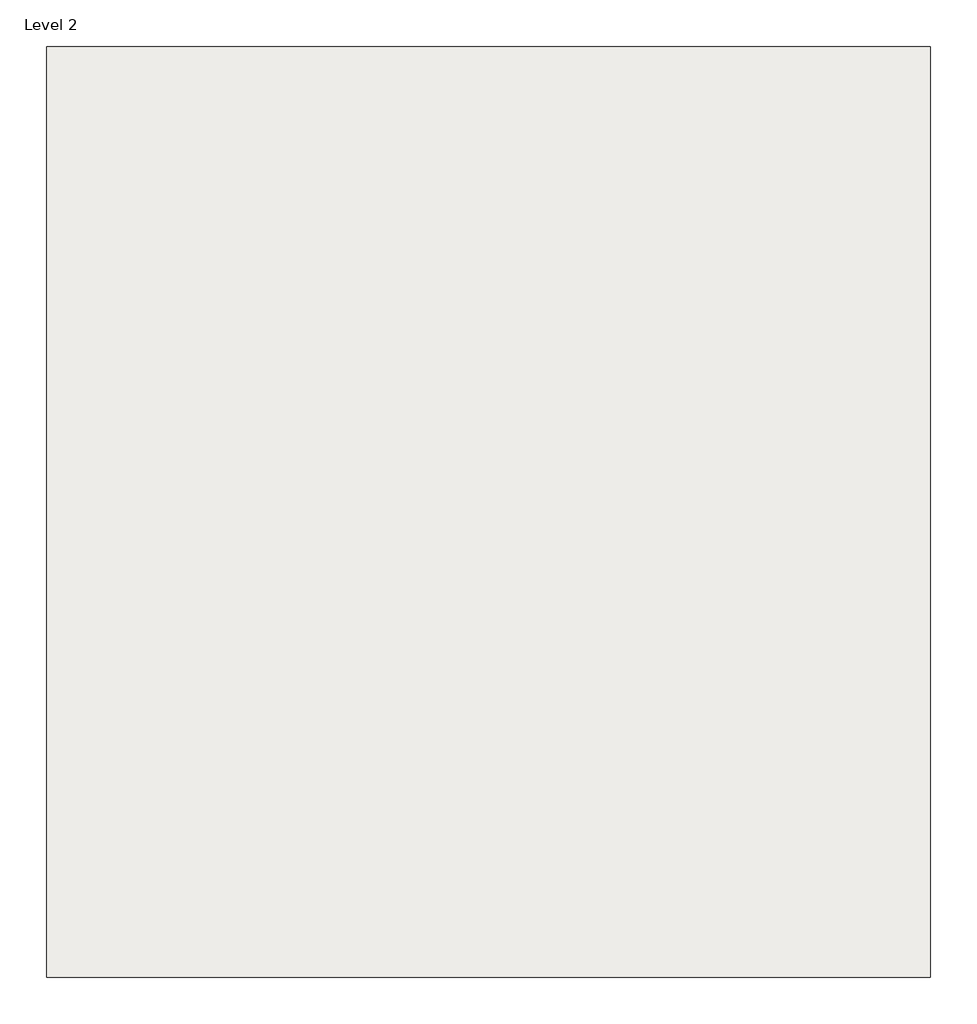
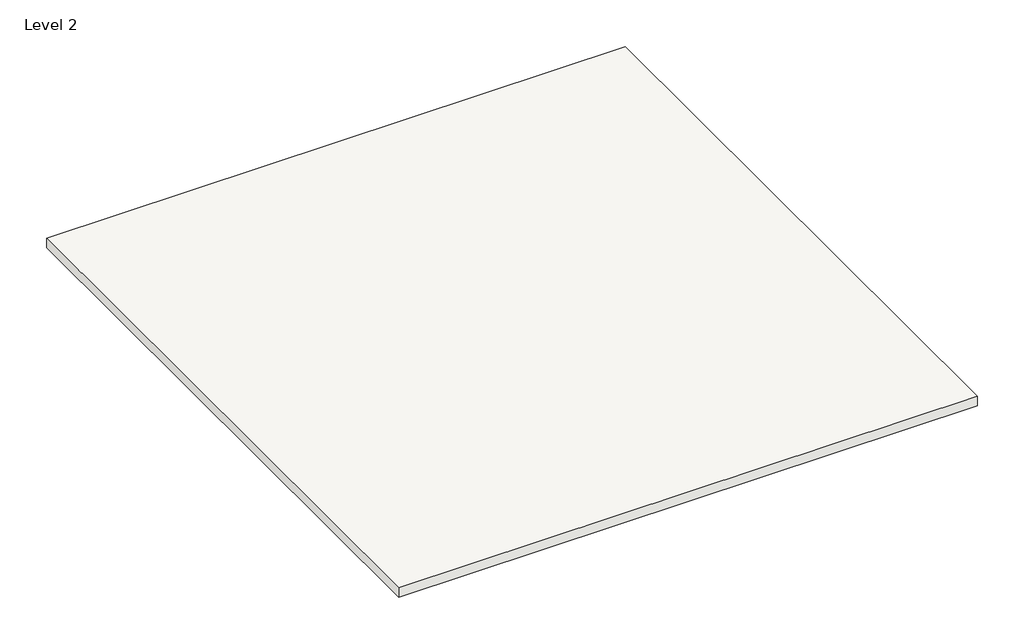
# One storey: 1 roof.
"""IFC4 building model written with IfcOpenShell, lengths in millimetres."""

from ifc_helpers import new_model, si_unit, frame, origin, place, context, project, spatial, polyline, outline, extrude, element, save

model = new_model("IFC4")

# Units and contexts
model_context = context("Model", 3, world=origin())
ifc_project = project(units=[si_unit("LENGTHUNIT", "METRE", prefix="MILLI")], contexts=[model_context])

# Site, building, storey
site = spatial("IfcSite", under=ifc_project)
building = spatial("IfcBuilding", under=site)
storey = spatial("IfcBuildingStorey", under=building, Name="Level 2", Elevation=3048.0)

# Roof
placement = place(None, origin())
element("IfcRoof", 1, ObjectType="Generic - 12\"", at=placement, inside=storey, context=model_context, shape_type="SweptSolid", body=[
    extrude(outline(polyline([(-9538.1097877, 18533.0307946), (4838.2902123, 18533.0307946), (4838.2902123, 3394.6307946), (-9538.1097877, 3394.6307946), (-9538.1097877, 18533.0307946)])), frame((0.0, 0.0, 3048.0), z_axis=(0.0, 0.0, 1.0), x_axis=(1.0, 0.0, 0.0)), (0.0, 0.0, 1.0), 243.8796875),
])

save(model, "model.ifc")

# Revit data of these elements
# Type "Generic - 12\""
#   Assembly Code = "B1020"
#   Layers, outside or top first: 0' - 9 77/128" no material (function 1)
# Element 1 (IfcRoof, "Generic - 12\"")
#   built-in parameter 1001705 = 10.8001 (stored number, unit not read)
#   built-in parameter 1001710 = 33615
#   Phase Created = New Construction
#   Materials on its faces: "Default Roof"
# Materials
#   "Default Roof": colour RGB 88 101 114, transparency 0
